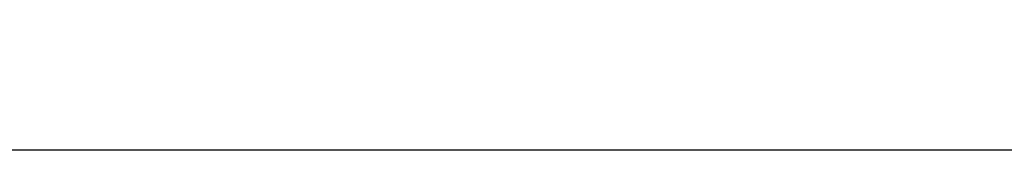
# Model space of a CAD drawing. Units: inches. Extents: x 1319 to 2030, y 219 to 1069.
# Tile 8 of 28: x 1506 to 1565, y 384 to 392. Entities that reach past the tile are written whole.
import ezdxf

# ---------------------------------------------------------------- set-up
doc = ezdxf.new("R2010")
doc.units = ezdxf.units.IN
doc.header["$MEASUREMENT"] = 0
doc.layers.add('A-ANNO-DIMS', color=2, linetype='Continuous', lineweight=18)
doc.styles.get("Standard").update_dxf_attribs({"font": 'arial.ttf'})
doc.dimstyles.get("Standard").update_dxf_attribs({"dimtxt": 7, "dimasz": 0.18, "dimexe": 0.18, "dimexo": 0.0625, "dimgap": 0.09, "dimtad": 0, "dimtih": 1, "dimtoh": 1, "dimzin": 0, "dimdsep": 46, "dimlunit": 3, "dimtxsty": 'Standard', "dimcen": 0.09, "dimadec": 0, "dimazin": 0, "dimtfac": 1, "dimtofl": 0, "dimtmove": 0, "dimatfit": 3, "dimfxl": 1, "dimtolj": 1, "dimtzin": 0, "dimarcsym": 0})

# ---------------------------------------------------------------- blocks, each defined once
blk = doc.blocks.new('*D65')
at = {"layer": 'A-ANNO-DIMS', "color": 0, "lineweight": -2, "transparency": 16777216}
for p, q in [((1648.280254, 472.227245), (1329.112754, 472.227245)), ((1329.292754, 472.047245), (1329.292754, 431.817245)), ((1329.292754, 384.407245), (1329.292754, 424.637245)), ((1648.280254, 384.227245), (1329.112754, 384.227245))]:
    blk.add_line(p, q, dxfattribs=at)
at = {"layer": 'A-ANNO-DIMS', "color": 0, "transparency": 16777216}
for points in [[(1329.262754, 472.047245), (1329.322754, 472.047245), (1329.292754, 472.227245)], [(1329.262754, 384.407245), (1329.322754, 384.407245), (1329.292754, 384.227245)]]:
    blk.add_solid(points, dxfattribs=at)
at = {"layer": 'Defpoints', "color": 0, "transparency": 16777216}
for p in [(1329.292754, 472.227245), (1648.342754, 472.227245), (1648.342754, 384.227245)]:
    blk.add_point(p, dxfattribs=at)
at = {"layer": 'A-ANNO-DIMS', "color": 0, "transparency": 16777216, "insert": (1329.292754, 428.227245), "char_height": 7, "attachment_point": 5}
blk.add_mtext('\\A1;7\'-4"', dxfattribs=at)

msp = doc.modelspace()

# ---------------------------------------------------------------- dimensions: what is measured, and where the dimension line sits
at = {"layer": 'A-ANNO-DIMS'}
dim = msp.add_linear_dim(base=(1329.293, 472.227), p1=(1648.343, 384.227), p2=(1648.343, 472.227), angle=90, dimstyle='Standard', override={"dimdec": 1, "dimlfac": 1, "dimrnd": 0, "dimzin": 1, "dimdsep": 46, "dimlunit": 4, "dimfrac": 2}, dxfattribs=at)
dim.commit()
dim.dimension.update_dxf_attribs({"geometry": '*D65', "text_midpoint": (1329.293, 428.227)})

doc.saveas('drawing.dxf')
